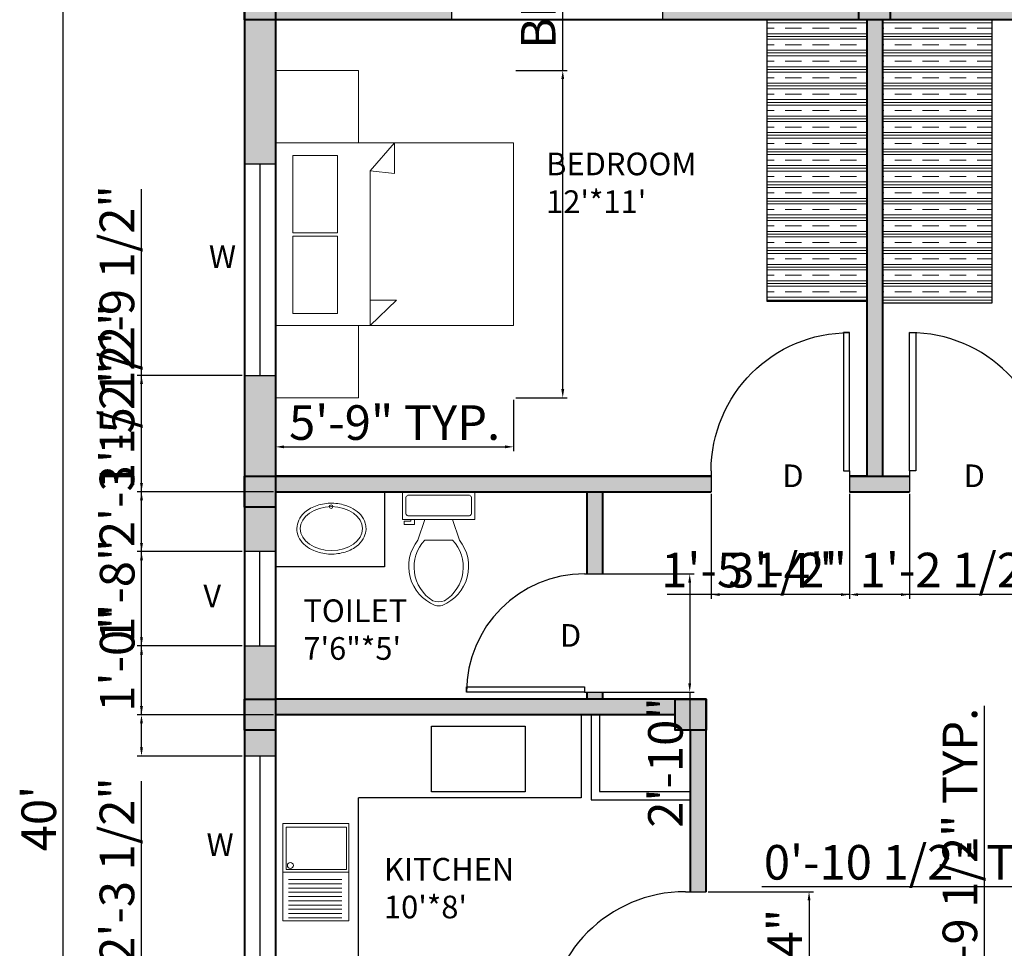
# Model space of a CAD drawing. Units: inches. Extents: x 1628 to 2197, y 2073 to 2736.
# Tile 2 of 3: x 1628 to 1913, y 2323 to 2592. Entities that reach past the tile are written whole.
import ezdxf

# ---------------------------------------------------------------- set-up
doc = ezdxf.new("R2010")
doc.units = ezdxf.units.IN
for name, color, linetype, lineweight in [('A-ANNO-DIMS', 2, 'Continuous', 18), ('A-ANNO-IDEN', 7, 'Continuous', 18), ('A-AREA-IDEN', 7, 'Continuous', 18), ('A-COLS', 7, 'Continuous', 40), ('A-COLS-PATT', 8, 'Continuous', 13), ('A-FLOR-CASE', 8, 'Continuous', 25), ('A-FLOR-CASE-PATT', 9, 'Continuous', 13), ('A-FLOR-FIXT', 8, 'Continuous', 18), ('A-FLOR-FIXT-PATT', 8, 'Continuous', 13), ('A-WALL-PATT', 152, 'Continuous', 13), ('bed', 210, 'Continuous', 18), ('door', 52, 'Continuous', 25), ('wall', 151, 'Continuous', 40), ('window', 20, 'Continuous', 25)]:
    doc.layers.add(name, color=color, linetype=linetype, lineweight=lineweight)
doc.styles.get("Standard").update_dxf_attribs({"font": 'arial.ttf'})
doc.dimstyles.new('ISO-25', dxfattribs={"dimtxt": 10, "dimasz": 2.5, "dimexe": 1.25, "dimexo": 0.625, "dimtad": 1, "dimdec": 0, "dimlunit": 4, "dimtxsty": 'Standard', "dimcen": 2.5, "dimadec": 0, "dimazin": 0, "dimtfac": 1, "dimtdec": 0, "dimtmove": 0, "dimatfit": 3, "dimfxl": 1, "dimarcsym": 0})

# ---------------------------------------------------------------- blocks, each defined once
blk = doc.blocks.new('*U2')
for p, q in [((0, 0), (-1e-16, -5.999999999999999)), ((40, -6e-16), (40, -6))]:
    blk.add_line(p, q)
blk.add_lwpolyline([(0, 0), (5.6e-15, 40), (1.750000000000007, 40), (1.749999999999998, -7e-16)], close=True)
blk.add_arc((0, 0), 40, 0, 90)
blk = doc.blocks.new('*U4')
for p, q in [((9.5, -6), (9.5, -2)), ((-10, -8.5), (-8, -8.5)), ((-10, -9.5), (-10, -8.5)), ((-8, -8.5), (-8, -8)), ((-7, -8), (-7, -9.5)), ((-4, -8), (-6, -14)), ((4, -8), (6, -14)), ((-7, -9.5), (-10, -9.5)), ((4, -14), (-4, -14))]:
    blk.add_line(p, q)
blk.add_lwpolyline([(10.5, -8), (10.5, 0), (-10.5, 0), (-10.5, -8)], close=True)
for points in [[(-9.5, -2), (-9.5, -6)], [(8.5, -1), (-8.5, -1)], [(-8.5, -7), (8.5, -7)]]:
    blk.add_lwpolyline(points)
for centre, radius, start, end in [((-8.625, -1.875), 0.8838834999999999, 81.86989999999999, 188.1300999999999), ((8.625, -1.875), 0.8838834999999999, 351.8699, 98.13009999999993), ((-8.625, -6.125), 0.8838834999999999, 171.869898, 278.1301), ((8.625, -6.125), 0.8838834999999999, 261.8699, 8.130099999999993), ((3.519562435188956, -21.58049502388982), 12.16902005083646, 141.4691096810948, 247.9714346835576), ((4.199957580658807, -21.81740929088453), 11.3291791325804, 136.3677254423718, 238.946823937405), ((-3.519499936778316, -21.58047137067522), 12.16903423757823, 292.0284332733152, 38.53070636800453), ((-4.199890672038477, -21.81738596564128), 11.32918622148567, 301.0530065773863, 43.63209216694732), ((2.09660981727e-05, -27.87646475467881), 4, 245.7318247449371, 294.2681740488959), ((2.09415214183e-05, -28.99996806116075), 4, 254.8605283244437, 285.1394707718433)]:
    blk.add_arc(centre, radius, start, end)
blk = doc.blocks.new('*D6')
at = {"layer": 'A-ANNO-DIMS', "color": 0, "lineweight": -2, "transparency": 16777216}
for p, q in [((1692.485896843686, 2600.702398616904), (1639.445355811252, 2600.702398616904)), ((1640.695355811253, 2123.202398616904), (1640.695355811252, 2598.202398616904)), ((1692.485896843686, 2120.702398616904), (1639.445355811253, 2120.702398616904))]:
    blk.add_line(p, q, dxfattribs=at)
at = {"layer": 'A-ANNO-DIMS', "color": 0, "transparency": 16777216}
for points in [[(1640.278689144586, 2598.202398616904), (1641.112022477919, 2598.202398616904), (1640.695355811252, 2600.702398616904)], [(1640.278689144586, 2123.202398616904), (1641.112022477919, 2123.202398616904), (1640.695355811253, 2120.702398616904)]]:
    blk.add_solid(points, dxfattribs=at)
at = {"layer": 'Defpoints', "color": 0, "transparency": 16777216}
for p in [(1640.695355811252, 2600.702398616904), (1693.110896843687, 2600.702398616904), (1693.110896843687, 2120.702398616904)]:
    blk.add_point(p, dxfattribs=at)
at = {"layer": 'A-ANNO-DIMS', "color": 0, "transparency": 16777216, "insert": (1634.964625934036, 2360.702398616903), "char_height": 10, "attachment_point": 5, "rotation": 90}
blk.add_mtext("40'", dxfattribs=at)
blk = doc.blocks.new('BED-DOUBLE-WITH-NIGHTSTANDS')
for p, q in [((27.36977918091793, 65.5958310632277), (34.42114521002327, 73.72468310128534)), ((34.42114521002327, 73.72468310128534), (34.42114521002327, 64.85614303712828)), ((27.36977918091793, 28.24148243144555), (27.36977918091793, 65.5958310632277)), ((34.42114521002327, 64.85614303712828), (27.36977918091793, 65.5958310632277)), ((27.36977918091793, 28.24148243144555), (27.36977918091793, 20.93786224134965)), ((27.36977918091793, 20.93786224134965), (34.95813081485972, 28.24148243144555)), ((34.95813081485972, 28.24148243144555), (27.36977918091793, 28.24148243144555))]:
    blk.add_line(p, q)
for points in [[(-0.0001031563144807, 73.72468310128534), (23.97928037784254, 73.72468310128534), (23.97928037784254, 94.66247624076277), (-0.0001031563144807, 94.66247624076277)], [(-0.0001031563144807, 20.93786224134965), (68.84239357636102, 20.93786224134965), (68.84239357636102, 73.72468310128534), (-0.0001031563144807, 73.72468310128534)], [(4.974907084450705, 47.65834800199082), (17.93062219200033, 47.65834800199082), (17.93062219200033, 70.03397213404423), (4.974907084450705, 70.03397213404423)], [(4.974907084450705, 24.35811060875858), (17.93062219200033, 24.35811060875858), (17.93062219200033, 46.73373474081199), (4.974907084450705, 46.73373474081199)], [(-0.0001031563144807, 6.91018722137e-05), (23.97928037784254, 6.91018722137e-05), (23.97928037784254, 20.93786224134965), (-0.0001031563144807, 20.93786224134965)]]:
    blk.add_lwpolyline(points, close=True)
blk = doc.blocks.new('WINDOW-61IN')
blk.add_line((-0.0003684333103138, 4.500398616903112), (61.10273973038352, 4.500398616903112))
blk.add_lwpolyline([(-0.0003684333103138, 0.0003986169031123), (61.10273973038352, 0.0003986169031123), (61.10273973038352, 9.000398616903112), (-0.0003684333103138, 9.000398616903112)], close=True)
blk = doc.blocks.new('COLUMN-9X9')
blk.add_lwpolyline([(-0.0001031563144807, 9.000398616903112), (8.99989684368552, 9.000398616903112), (8.99989684368552, 0.0003986169031123), (-0.0001031563144807, 0.0003986169031123)], close=True)
blk = doc.blocks.new('*D18')
at = {"layer": 'A-ANNO-DIMS', "color": 0, "lineweight": -2, "transparency": 16777216}
for p, q in [((1938.501053468832, 2340.938171535931), (1842.725132595708, 2340.938171535927)), ((1938.501053468832, 2342.288259422146), (1938.501053468832, 2339.688171535931)), ((1946.605665621899, 2340.938171535931), (1941.001053468832, 2340.938171535931)), ((1949.1056656219, 2342.288259422147), (1949.1056656219, 2339.688171535931))]:
    blk.add_line(p, q, dxfattribs=at)
at = {"layer": 'A-ANNO-DIMS', "color": 0, "transparency": 16777216}
for points in [[(1941.001053468832, 2341.354838202597), (1941.001053468832, 2340.521504869264), (1938.501053468832, 2340.938171535931)], [(1946.605665621899, 2341.354838202597), (1946.605665621899, 2340.521504869264), (1949.1056656219, 2340.938171535931)]]:
    blk.add_solid(points, dxfattribs=at)
at = {"layer": 'Defpoints', "color": 0, "transparency": 16777216}
for p in [(1938.501053468832, 2342.913259422146), (1949.1056656219, 2342.913259422147), (1938.501053468832, 2340.938171535931)]:
    blk.add_point(p, dxfattribs=at)
at = {"layer": 'A-ANNO-DIMS', "color": 0, "transparency": 16777216, "insert": (1889.36309303227, 2346.733703595956), "char_height": 10, "attachment_point": 5}
blk.add_mtext('0\'-10 1/2" TYP.', dxfattribs=at)
blk = doc.blocks.new('*D19')
at = {"layer": 'A-ANNO-DIMS', "color": 0, "lineweight": -2, "transparency": 16777216}
for p, q in [((1785.152754647198, 2577.035625777927), (1785.152754647198, 2736.024370661965)), ((1771.578393576364, 2577.035625777927), (1786.402754647198, 2577.035625777927)), ((1785.152754647198, 2484.873218639036), (1785.152754647198, 2574.535625777927)), ((1771.578393576364, 2482.373218639037), (1786.402754647198, 2482.373218639037))]:
    blk.add_line(p, q, dxfattribs=at)
at = {"layer": 'A-ANNO-DIMS', "color": 0, "transparency": 16777216}
for points in [[(1784.736087980531, 2574.535625777927), (1785.569421313865, 2574.535625777927), (1785.152754647198, 2577.035625777927)], [(1784.736087980532, 2484.873218639036), (1785.569421313865, 2484.873218639036), (1785.152754647198, 2482.373218639037)]]:
    blk.add_solid(points, dxfattribs=at)
at = {"layer": 'Defpoints', "color": 0, "transparency": 16777216}
for p in [(1770.953393576364, 2577.035625777927), (1785.152754647198, 2577.035625777927), (1770.953393576364, 2482.373218639037)]:
    blk.add_point(p, dxfattribs=at)
at = {"layer": 'A-ANNO-DIMS', "color": 0, "transparency": 16777216, "insert": (1779.357222587171, 2657.779998219945), "char_height": 10, "attachment_point": 5, "rotation": 90}
blk.add_mtext('BED SET 7\'-10 1/2" TYP.', dxfattribs=at)
blk = doc.blocks.new('*D20')
at = {"layer": 'A-ANNO-DIMS', "color": 0, "lineweight": -2, "transparency": 16777216}
for p, q in [((1702.110896843687, 2481.748218639035), (1702.110896843687, 2466.923857568202)), ((1770.953393576363, 2481.748218639035), (1770.953393576363, 2466.923857568202)), ((1704.610896843687, 2468.173857568201), (1768.453393576363, 2468.173857568201))]:
    blk.add_line(p, q, dxfattribs=at)
at = {"layer": 'A-ANNO-DIMS', "color": 0, "transparency": 16777216}
for points in [[(1704.610896843687, 2468.590524234868), (1704.610896843687, 2467.757190901535), (1702.110896843687, 2468.173857568201)], [(1768.453393576363, 2468.590524234868), (1768.453393576363, 2467.757190901535), (1770.953393576363, 2468.173857568201)]]:
    blk.add_solid(points, dxfattribs=at)
at = {"layer": 'Defpoints', "color": 0, "transparency": 16777216}
for p in [(1702.110896843687, 2482.373218639035), (1770.953393576363, 2482.373218639035), (1770.953393576363, 2468.173857568201)]:
    blk.add_point(p, dxfattribs=at)
at = {"layer": 'A-ANNO-DIMS', "color": 0, "transparency": 16777216, "insert": (1736.532145210025, 2473.904587445419), "char_height": 10, "attachment_point": 5}
blk.add_mtext('5\'-9" TYP.', dxfattribs=at)
blk = doc.blocks.new('*D24')
at = {"layer": 'A-ANNO-DIMS', "color": 0, "lineweight": -2, "transparency": 16777216}
for p, q in [((1907.071103678795, 2305.097810115476), (1907.071103678795, 2393.274822393784)), ((1916.945934926503, 2305.097810115476), (1905.821103678795, 2305.097810115476)), ((1907.071103678795, 2274.241064235891), (1907.071103678795, 2302.597810115477)), ((1916.945934926503, 2271.741064235891), (1905.821103678795, 2271.741064235891))]:
    blk.add_line(p, q, dxfattribs=at)
at = {"layer": 'A-ANNO-DIMS', "color": 0, "transparency": 16777216}
for points in [[(1906.654437012129, 2302.597810115477), (1907.487770345462, 2302.597810115477), (1907.071103678795, 2305.097810115476)], [(1906.654437012129, 2274.241064235891), (1907.487770345462, 2274.241064235891), (1907.071103678795, 2271.741064235891)]]:
    blk.add_solid(points, dxfattribs=at)
at = {"layer": 'Defpoints', "color": 0, "transparency": 16777216}
for p in [(1907.071103678795, 2305.097810115476), (1917.570934926503, 2305.097810115476), (1917.570934926503, 2271.741064235891)]:
    blk.add_point(p, dxfattribs=at)
at = {"layer": 'A-ANNO-DIMS', "color": 0, "transparency": 16777216, "insert": (1901.275571618768, 2350.43631625463), "char_height": 10, "attachment_point": 5, "rotation": 90}
blk.add_mtext('2\'-9 1/2" TYP.', dxfattribs=at)
blk = doc.blocks.new('*D35')
at = {"layer": 'A-ANNO-DIMS', "color": 0, "lineweight": -2, "transparency": 16777216}
for p, q in [((1663.360897000002, 2317.649085000001), (1663.360897000002, 2371.45365525921)), ((1692.485897000001, 2317.649085000001), (1662.110897000002, 2317.649085000001)), ((1663.360897000002, 2292.702399000001), (1663.360897000002, 2315.149085000001)), ((1701.485897000001, 2290.202399000001), (1662.110897000002, 2290.202399000001))]:
    blk.add_line(p, q, dxfattribs=at)
at = {"layer": 'A-ANNO-DIMS', "color": 0, "transparency": 16777216}
for points in [[(1662.944230333335, 2315.149085000001), (1663.777563666668, 2315.149085000001), (1663.360897000002, 2317.649085000001)], [(1662.944230333335, 2292.702399000001), (1663.777563666668, 2292.702399000001), (1663.360897000002, 2290.202399000001)]]:
    blk.add_solid(points, dxfattribs=at)
at = {"layer": 'Defpoints', "color": 0, "transparency": 16777216}
for p in [(1663.360897000002, 2317.649085000001), (1693.110897000001, 2317.649085000001), (1702.110897000001, 2290.202399000001)]:
    blk.add_point(p, dxfattribs=at)
at = {"layer": 'A-ANNO-DIMS', "color": 0, "transparency": 16777216, "insert": (1657.561954298774, 2345.801370129604), "char_height": 10, "attachment_point": 5, "rotation": 90}
blk.add_mtext('2\'-3 1/2"', dxfattribs=at)
blk = doc.blocks.new('*D36')
at = {"layer": 'A-ANNO-DIMS', "color": 0, "lineweight": -2, "transparency": 16777216}
for p, q in [((1663.360897000002, 2390.702399000001), (1663.360897000002, 2420.093599545703)), ((1701.485897000001, 2390.702399000001), (1662.110897000002, 2390.702399000001)), ((1663.360897000002, 2381.252193000001), (1663.360897000002, 2388.202399000001)), ((1692.485897000001, 2378.752193000001), (1662.110897000002, 2378.752193000001))]:
    blk.add_line(p, q, dxfattribs=at)
at = {"layer": 'A-ANNO-DIMS', "color": 0, "transparency": 16777216}
for points in [[(1662.944230333335, 2388.202399000001), (1663.777563666668, 2388.202399000001), (1663.360897000002, 2390.702399000001)], [(1662.944230333335, 2381.252193000001), (1663.777563666668, 2381.252193000001), (1663.360897000002, 2378.752193000001)]]:
    blk.add_solid(points, dxfattribs=at)
at = {"layer": 'Defpoints', "color": 0, "transparency": 16777216}
for p in [(1663.360897000002, 2390.702399000001), (1702.110897000001, 2390.702399000001), (1693.110897000001, 2378.752193000001)]:
    blk.add_point(p, dxfattribs=at)
at = {"layer": 'A-ANNO-DIMS', "color": 0, "transparency": 16777216, "insert": (1657.630167122785, 2406.647999272851), "char_height": 10, "attachment_point": 5, "rotation": 90}
blk.add_mtext('1\'-0"', dxfattribs=at)
blk = doc.blocks.new('*D37')
at = {"layer": 'A-ANNO-DIMS', "color": 0, "lineweight": -2, "transparency": 16777216}
for p, q in [((1663.360897000002, 2410.599066000001), (1663.360897000002, 2439.990266545704)), ((1692.485897000001, 2410.599066000001), (1662.110897000002, 2410.599066000001)), ((1663.360897000002, 2393.202399000001), (1663.360897000002, 2408.099066000001)), ((1701.485897000001, 2390.702399000001), (1662.110897000002, 2390.702399000001))]:
    blk.add_line(p, q, dxfattribs=at)
at = {"layer": 'A-ANNO-DIMS', "color": 0, "transparency": 16777216}
for points in [[(1662.944230333335, 2408.099066000001), (1663.777563666668, 2408.099066000001), (1663.360897000002, 2410.599066000001)], [(1662.944230333335, 2393.202399000001), (1663.777563666668, 2393.202399000001), (1663.360897000002, 2390.702399000001)]]:
    blk.add_solid(points, dxfattribs=at)
at = {"layer": 'Defpoints', "color": 0, "transparency": 16777216}
for p in [(1663.360897000002, 2410.599066000001), (1693.110897000001, 2410.599066000001), (1702.110897000001, 2390.702399000001)]:
    blk.add_point(p, dxfattribs=at)
at = {"layer": 'A-ANNO-DIMS', "color": 0, "transparency": 16777216, "insert": (1657.630167122785, 2426.544666272852), "char_height": 10, "attachment_point": 5, "rotation": 90}
blk.add_mtext('1\'-8"', dxfattribs=at)
blk = doc.blocks.new('*D38')
at = {"layer": 'A-ANNO-DIMS', "color": 0, "lineweight": -2, "transparency": 16777216}
for p, q in [((1663.360897000002, 2437.863608000001), (1663.360897000002, 2491.66817825921)), ((1692.485897000001, 2437.863608000001), (1662.110897000002, 2437.863608000001)), ((1663.360897000002, 2413.099066000001), (1663.360897000002, 2435.363608000001)), ((1692.485897000001, 2410.599066000001), (1662.110897000002, 2410.599066000001))]:
    blk.add_line(p, q, dxfattribs=at)
at = {"layer": 'A-ANNO-DIMS', "color": 0, "transparency": 16777216}
for points in [[(1662.944230333335, 2435.363608000001), (1663.777563666668, 2435.363608000001), (1663.360897000002, 2437.863608000001)], [(1662.944230333335, 2413.099066000001), (1663.777563666668, 2413.099066000001), (1663.360897000002, 2410.599066000001)]]:
    blk.add_solid(points, dxfattribs=at)
at = {"layer": 'Defpoints', "color": 0, "transparency": 16777216}
for p in [(1663.360897000002, 2437.863608000001), (1693.110897000001, 2437.863608000001), (1693.110897000001, 2410.599066000001)]:
    blk.add_point(p, dxfattribs=at)
at = {"layer": 'A-ANNO-DIMS', "color": 0, "transparency": 16777216, "insert": (1657.561954298774, 2466.015893129605), "char_height": 10, "attachment_point": 5, "rotation": 90}
blk.add_mtext('2\'-3 1/2"', dxfattribs=at)
blk = doc.blocks.new('*D39')
at = {"layer": 'A-ANNO-DIMS', "color": 0, "lineweight": -2, "transparency": 16777216}
for p, q in [((1663.360897000002, 2455.202399000001), (1663.360897000002, 2507.895100227831)), ((1701.485897000001, 2455.202399000001), (1662.110897000002, 2455.202399000001)), ((1663.360897000002, 2440.363608000001), (1663.360897000002, 2452.702399000001)), ((1692.485897000001, 2437.863608000001), (1662.110897000002, 2437.863608000001))]:
    blk.add_line(p, q, dxfattribs=at)
at = {"layer": 'A-ANNO-DIMS', "color": 0, "transparency": 16777216}
for points in [[(1662.944230333335, 2452.702399000001), (1663.777563666668, 2452.702399000001), (1663.360897000002, 2455.202399000001)], [(1662.944230333335, 2440.363608000001), (1663.777563666668, 2440.363608000001), (1663.360897000002, 2437.863608000001)]]:
    blk.add_solid(points, dxfattribs=at)
at = {"layer": 'Defpoints', "color": 0, "transparency": 16777216}
for p in [(1663.360897000002, 2455.202399000001), (1702.110897000001, 2455.202399000001), (1693.110897000001, 2437.863608000001)]:
    blk.add_point(p, dxfattribs=at)
at = {"layer": 'A-ANNO-DIMS', "color": 0, "transparency": 16777216, "insert": (1657.565364939975, 2482.798749613916), "char_height": 10, "attachment_point": 5, "rotation": 90}
blk.add_mtext('1\'-5 1/2"', dxfattribs=at)
blk = doc.blocks.new('*D40')
at = {"layer": 'A-ANNO-DIMS', "color": 0, "lineweight": -2, "transparency": 16777216}
for p, q in [((1663.360897000002, 2488.850109000001), (1663.360897000002, 2542.65467925921)), ((1692.485897000001, 2488.850109000001), (1662.110897000002, 2488.850109000001)), ((1663.360897000002, 2457.702399000001), (1663.360897000002, 2486.350109000001)), ((1701.485897000001, 2455.202399000001), (1662.110897000002, 2455.202399000001))]:
    blk.add_line(p, q, dxfattribs=at)
at = {"layer": 'A-ANNO-DIMS', "color": 0, "transparency": 16777216}
for points in [[(1662.944230333335, 2486.350109000001), (1663.777563666668, 2486.350109000001), (1663.360897000002, 2488.850109000001)], [(1662.944230333335, 2457.702399000001), (1663.777563666668, 2457.702399000001), (1663.360897000002, 2455.202399000001)]]:
    blk.add_solid(points, dxfattribs=at)
at = {"layer": 'Defpoints', "color": 0, "transparency": 16777216}
for p in [(1663.360897000002, 2488.850109000001), (1693.110897000001, 2488.850109000001), (1702.110897000001, 2455.202399000001)]:
    blk.add_point(p, dxfattribs=at)
at = {"layer": 'A-ANNO-DIMS', "color": 0, "transparency": 16777216, "insert": (1657.565364939975, 2517.002394129605), "char_height": 10, "attachment_point": 5, "rotation": 90}
blk.add_mtext('2\'-9 1/2"', dxfattribs=at)
blk = doc.blocks.new('*D48')
at = {"layer": 'A-ANNO-DIMS', "color": 0, "lineweight": -2, "transparency": 16777216}
for p, q in [((1792.735897000001, 2431.437917000002), (1823.110897000002, 2431.437917000002)), ((1821.860897000002, 2428.937917000001), (1821.860897000002, 2399.766059000001)), ((1792.735897000001, 2397.266059000001), (1823.110897000002, 2397.266059000001)), ((1821.860897000002, 2397.266059000001), (1821.860897000002, 2358.993548768077))]:
    blk.add_line(p, q, dxfattribs=at)
at = {"layer": 'A-ANNO-DIMS', "color": 0, "transparency": 16777216}
for points in [[(1821.444230333335, 2428.937917000001), (1822.277563666668, 2428.937917000001), (1821.860897000002, 2431.437917000002)], [(1821.444230333335, 2399.766059000001), (1822.277563666668, 2399.766059000001), (1821.860897000002, 2397.266059000001)]]:
    blk.add_solid(points, dxfattribs=at)
at = {"layer": 'Defpoints', "color": 0, "transparency": 16777216}
for p in [(1792.110897000001, 2431.437917000002), (1792.110897000001, 2397.266059000001), (1821.860897000002, 2397.266059000001)]:
    blk.add_point(p, dxfattribs=at)
at = {"layer": 'A-ANNO-DIMS', "color": 0, "transparency": 16777216, "insert": (1816.130167122785, 2376.879803884039), "char_height": 10, "attachment_point": 5, "rotation": 90}
blk.add_mtext('2\'-10"', dxfattribs=at)
blk = doc.blocks.new('*D49')
at = {"layer": 'A-ANNO-DIMS', "color": 0, "lineweight": -2, "transparency": 16777216}
for p, q in [((1828.052739, 2454.577399), (1828.052739, 2424.202399)), ((1868.052739, 2454.577399), (1868.052739, 2424.202399)), ((1865.552739, 2425.452399), (1830.552739, 2425.452399))]:
    blk.add_line(p, q, dxfattribs=at)
at = {"layer": 'A-ANNO-DIMS', "color": 0, "transparency": 16777216}
for points in [[(1830.552739, 2425.869065666666), (1830.552739, 2425.035732333333), (1828.052739, 2425.452399)], [(1865.552739, 2425.869065666666), (1865.552739, 2425.035732333333), (1868.052739, 2425.452399)]]:
    blk.add_solid(points, dxfattribs=at)
at = {"layer": 'Defpoints', "color": 0, "transparency": 16777216}
for p in [(1828.052739, 2455.202399), (1868.052739, 2455.202399), (1828.052739, 2425.452399)]:
    blk.add_point(p, dxfattribs=at)
at = {"layer": 'A-ANNO-DIMS', "color": 0, "transparency": 16777216, "insert": (1848.052739, 2431.186539518418), "char_height": 10, "attachment_point": 5}
blk.add_mtext('3\'-4"', dxfattribs=at)
blk = doc.blocks.new('*D50')
at = {"layer": 'A-ANNO-DIMS', "color": 0, "lineweight": -2, "transparency": 16777216}
for p, q in [((1868.052739, 2454.577399), (1868.052739, 2424.202399)), ((1885.432438, 2454.577399), (1885.432438, 2424.202399)), ((1868.052739, 2425.452399), (1815.360037772169, 2425.452399)), ((1882.932438, 2425.452399), (1870.552739, 2425.452399))]:
    blk.add_line(p, q, dxfattribs=at)
at = {"layer": 'A-ANNO-DIMS', "color": 0, "transparency": 16777216}
for points in [[(1870.552739, 2425.869065666666), (1870.552739, 2425.035732333333), (1868.052739, 2425.452399)], [(1882.932438, 2425.869065666666), (1882.932438, 2425.035732333333), (1885.432438, 2425.452399)]]:
    blk.add_solid(points, dxfattribs=at)
at = {"layer": 'Defpoints', "color": 0, "transparency": 16777216}
for p in [(1868.052739, 2455.202399), (1885.432438, 2455.202399), (1868.052739, 2425.452399)]:
    blk.add_point(p, dxfattribs=at)
at = {"layer": 'A-ANNO-DIMS', "color": 0, "transparency": 16777216, "insert": (1840.456388386084, 2431.247931060027), "char_height": 10, "attachment_point": 5}
blk.add_mtext('1\'-5 1/2"', dxfattribs=at)
blk = doc.blocks.new('*D51')
at = {"layer": 'A-ANNO-DIMS', "color": 0, "lineweight": -2, "transparency": 16777216}
for p, q in [((1925.432438, 2454.577399), (1925.432437999998, 2424.202399)), ((1940.110897, 2454.577399), (1940.110896999998, 2424.202398999999)), ((1925.432437999998, 2425.452399), (1872.739736772167, 2425.452399000004)), ((1937.610896999998, 2425.452399), (1927.932437999998, 2425.452399))]:
    blk.add_line(p, q, dxfattribs=at)
at = {"layer": 'A-ANNO-DIMS', "color": 0, "transparency": 16777216}
for points in [[(1927.932437999998, 2425.869065666666), (1927.932437999998, 2425.035732333333), (1925.432437999998, 2425.452399)], [(1937.610896999998, 2425.869065666666), (1937.610896999998, 2425.035732333333), (1940.110896999998, 2425.452399)]]:
    blk.add_solid(points, dxfattribs=at)
at = {"layer": 'Defpoints', "color": 0, "transparency": 16777216}
for p in [(1925.432438, 2455.202399), (1940.110897, 2455.202399), (1925.432437999998, 2425.452399)]:
    blk.add_point(p, dxfattribs=at)
at = {"layer": 'A-ANNO-DIMS', "color": 0, "transparency": 16777216, "insert": (1897.836087386083, 2431.247931060029), "char_height": 10, "attachment_point": 5}
blk.add_mtext('1\'-2 1/2"', dxfattribs=at)
blk = doc.blocks.new('*D53')
at = {"layer": 'A-ANNO-DIMS', "color": 0, "lineweight": -2, "transparency": 16777216}
for p, q in [((1827.235897000001, 2339.518037000001), (1857.610897000002, 2339.518037000001)), ((1856.360897000002, 2337.018037000001), (1856.360897000002, 2302.018037000001)), ((1827.235897000001, 2299.518037000001), (1857.610897000002, 2299.518037000001))]:
    blk.add_line(p, q, dxfattribs=at)
at = {"layer": 'A-ANNO-DIMS', "color": 0, "transparency": 16777216}
for points in [[(1855.944230333335, 2337.018037000001), (1856.777563666668, 2337.018037000001), (1856.360897000002, 2339.518037000001)], [(1855.944230333335, 2302.018037000001), (1856.777563666668, 2302.018037000001), (1856.360897000002, 2299.518037000001)]]:
    blk.add_solid(points, dxfattribs=at)
at = {"layer": 'Defpoints', "color": 0, "transparency": 16777216}
for p in [(1826.610897000001, 2339.518037000001), (1826.610897000001, 2299.518037000001), (1856.360897000002, 2299.518037000001)]:
    blk.add_point(p, dxfattribs=at)
at = {"layer": 'A-ANNO-DIMS', "color": 0, "transparency": 16777216, "insert": (1850.626756481585, 2319.518037), "char_height": 10, "attachment_point": 5, "rotation": 90}
blk.add_mtext('3\'-4"', dxfattribs=at)

msp = doc.modelspace()

# ---------------------------------------------------------------- hatches: boundary and pattern name
at = {"layer": 'A-COLS-PATT'}
h = msp.add_hatch(color=256, dxfattribs=at)
h.dxf.hatch_style = 1
h.paths.add_polyline_path([(1702.110896843685, 2600.702398616903), (1693.110896843685, 2600.702398616903), (1693.110896843685, 2591.702398616904), (1702.110896843685, 2591.702398616904)])
h.paths.add_polyline_path([(1879.789544656754, 2600.702398616903), (1870.789544656754, 2600.702398616903), (1870.789544656754, 2591.702398616904), (1879.789544656754, 2591.702398616904)])
h.paths.add_polyline_path([(2053.110896843686, 2600.702398616903), (2044.110896843686, 2600.702398616903), (2044.110896843686, 2591.702398616904), (2053.110896843686, 2591.702398616904)])
h.paths.add_polyline_path([(1702.110896843685, 2395.202398616904), (1693.110896843685, 2395.202398616904), (1693.110896843685, 2386.202398616903), (1702.110896843685, 2386.202398616903)])
h.paths.add_polyline_path([(1826.610896843686, 2395.202398616904), (1817.610896843685, 2395.202398616904), (1817.610896843685, 2386.202398616903), (1826.610896843686, 2386.202398616903)])
h.paths.add_polyline_path([(1702.110896843685, 2459.702398616903), (1693.110896843685, 2459.702398616903), (1693.110896843685, 2450.702398616904), (1702.110896843685, 2450.702398616904)])
h.paths.add_polyline_path([(2053.110896843686, 2459.702398616903), (2044.110896843686, 2459.702398616903), (2044.110896843686, 2455.202398616903), (2053.110896843686, 2455.202398616903)])
h.paths.add_polyline_path([(2053.110896843686, 2455.202398616903), (2044.110896843686, 2455.202398616903), (2044.110896843686, 2451.940390996), (2053.110896843686, 2451.940390996)])
h.paths.add_polyline_path([(2053.110896843686, 2460.940390996), (2044.110896843686, 2460.940390996), (2044.110896843686, 2459.702398616903), (2053.110896843686, 2459.702398616903)])
h.paths.add_polyline_path([(2053.110896843686, 2390.990533735672), (2044.110896843686, 2390.990533735672), (2044.110896843686, 2381.990533735671), (2053.110896843686, 2381.990533735671)])
h.paths.add_polyline_path([(2053.110896843686, 2322.517334083322), (2044.110896843686, 2322.517334083322), (2044.110896843686, 2313.517334083321), (2053.110896843686, 2313.517334083321)])
h.paths.add_polyline_path([(1702.110896843685, 2294.702398616903), (1693.110896843685, 2294.702398616903), (1693.110896843685, 2285.702398616903), (1702.110896843685, 2285.702398616903)])
h.paths.add_polyline_path([(1702.110896843685, 2129.702398616903), (1693.110896843685, 2129.702398616903), (1693.110896843685, 2120.702398616904), (1702.110896843685, 2120.702398616904)])
h.paths.add_polyline_path([(1831.350600622014, 2129.702398616903), (1822.350600622014, 2129.702398616903), (1822.350600622014, 2120.702398616904), (1831.350600622014, 2120.702398616904)])
h.paths.add_polyline_path([(1883.720266620277, 2129.702398616903), (1874.720266620277, 2129.702398616903), (1874.720266620277, 2120.702398616904), (1883.720266620277, 2120.702398616904)])
h.paths.add_polyline_path([(2053.110896843686, 2129.702398616903), (2044.110896843686, 2129.702398616903), (2044.110896843686, 2120.702398616904), (2053.110896843686, 2120.702398616904)])
at = {"layer": 'A-FLOR-CASE-PATT'}
h = msp.add_hatch(dxfattribs=at)
h.set_pattern_fill('CLAY', color=256)
h.set_pattern_definition([(0, (0, 0), (0, 4.7625), []), (0, (0, 0.79375), (0, 4.7625), []), (0, (0, 1.587499999999999), (0, 4.7625), []), (0, (0, 3.174999999999999), (0, 4.7625), [4.7625, -3.174999999999999])])
h.paths.add_polyline_path([(1873.110896843686, 2591.702398616904), (1844.252398980434, 2591.702398616904), (1844.252398980434, 2510.242728136783), (1873.110896843686, 2510.242728136783)])
h.paths.add_polyline_path([(1909.320134716665, 2591.702398616904), (1877.610896843685, 2591.702398616904), (1877.610896843685, 2509.82863999123), (1909.320134716665, 2509.82863999123)])
at = {"layer": 'A-FLOR-FIXT-PATT'}
h = msp.add_hatch(dxfattribs=at)
h.set_pattern_fill('ANSI31', color=256, scale=0.386166, angle=-45, style=0)
h.set_pattern_definition([(0, (0, 0), (0, 1.22607705), [])])
h.paths.add_polyline_path([(1705.896944, 2331.99642), (1721.236081, 2331.99642), (1721.236081, 2344.176245), (1705.896944, 2344.176245)])
at = {"layer": 'A-WALL-PATT'}
h = msp.add_hatch(color=256, dxfattribs=at)
h.dxf.hatch_style = 1
h.paths.add_polyline_path([(1753.013631566689, 2600.702398616903), (1702.110896843685, 2600.702398616903), (1702.110896843685, 2591.702398616904), (1753.013631566689, 2591.702398616904)])
h.paths.add_polyline_path([(1870.789544656754, 2600.702398616903), (1814.116739730383, 2600.702398616903), (1814.116739730383, 2591.702398616904), (1870.789544656754, 2591.702398616904)])
h.paths.add_polyline_path([(1948.368746460448, 2600.702398616903), (1879.789544656754, 2600.702398616903), (1879.789544656754, 2591.702398616904), (1909.320134716665, 2591.702398616904), (1948.368746460448, 2591.702398616904)])
h.paths.add_polyline_path([(2044.110896843686, 2600.702398616903), (2009.471854624142, 2600.702398616903), (2009.471854624142, 2591.702398616904), (2044.110896843686, 2591.702398616904)])
h.paths.add_polyline_path([(2053.110896843686, 2591.702398616904), (2044.110896843686, 2591.702398616904), (2044.110896843686, 2550.072421842385), (2053.110896843686, 2550.072421842385)])
h.paths.add_polyline_path([(1702.110896843685, 2591.702398616904), (1693.110896843685, 2591.702398616904), (1693.110896843685, 2549.953217094844), (1702.110896843685, 2549.953217094844)])
h.paths.add_polyline_path([(1702.110896843685, 2488.85010893115), (1693.110896843685, 2488.85010893115), (1693.110896843685, 2459.702398616903), (1702.110896843685, 2459.702398616903)])
h.paths.add_polyline_path([(1828.052739298115, 2459.702398616904), (1702.110896843685, 2459.702398616903), (1702.110896843685, 2455.202398616903), (1733.607219099031, 2455.202398616903), (1792.110896843686, 2455.202398616903), (1828.052739298115, 2455.202398616904)])
h.paths.add_polyline_path([(1885.432437777228, 2459.702398616904), (1868.052739298114, 2459.702398616904), (1868.052739298114, 2455.202398616904), (1885.432437777228, 2455.202398616904)])
h.paths.add_polyline_path([(2053.110896843686, 2488.969313678691), (2044.110896843686, 2488.969313678691), (2044.110896843686, 2474.676024548712), (2044.110896843686, 2460.940390996), (2053.110896843686, 2460.940390996)])
h.paths.add_polyline_path([(2053.110896843686, 2451.940390996), (2044.110896843686, 2451.940390996), (2044.110896843686, 2437.286361970541), (2053.110896843686, 2437.286361970541)])
h.paths.add_polyline_path([(2053.110896843686, 2414.882591286594), (2044.110896843686, 2414.882591286594), (2044.110896843686, 2390.990533735672), (2053.110896843686, 2390.990533735672)])
h.paths.add_polyline_path([(2044.110896843686, 2459.702398616903), (1925.432437777228, 2459.702398616904), (1925.432437777228, 2455.202398616904), (2044.110896843686, 2455.202398616903)])
h.paths.add_polyline_path([(2053.110896843686, 2381.990533735671), (2044.110896843686, 2381.990533735671), (2044.110896843686, 2322.517334083322), (2053.110896843686, 2322.517334083322)])
h.paths.add_polyline_path([(1919.510741842323, 2129.702398616903), (1883.720266620277, 2129.702398616903), (1883.720266620277, 2120.702398616904), (1919.510741842323, 2120.702398616904)])
h.paths.add_polyline_path([(2044.110896843686, 2129.702398616903), (1980.613850006017, 2129.702398616903), (1980.613850006017, 2120.702398616904), (2044.110896843686, 2120.702398616904)])
h.paths.add_polyline_path([(2053.110896843686, 2207.91287215655), (2044.110896843686, 2207.91287215655), (2044.110896843686, 2129.702398616903), (2053.110896843686, 2129.702398616903)])
h.paths.add_polyline_path([(2053.110896843686, 2313.517334083321), (2044.110896843686, 2313.517334083321), (2044.110896843686, 2269.015980320244), (2053.110896843686, 2269.015980320244)])
h.paths.add_polyline_path([(1822.350600622014, 2129.702398616903), (1785.245011413373, 2129.702398616903), (1785.245011413373, 2120.702398616904), (1822.350600622014, 2120.702398616904)])
h.paths.add_polyline_path([(1724.14190324968, 2129.702398616903), (1702.110896843685, 2129.702398616903), (1702.110896843685, 2120.702398616904), (1724.14190324968, 2120.702398616904)])
h.paths.add_polyline_path([(1702.110896843685, 2168.735790533592), (1693.110896843685, 2168.735790533592), (1693.110896843685, 2129.702398616903), (1702.110896843685, 2129.702398616903)])
h.paths.add_polyline_path([(1702.110896843685, 2285.702398616903), (1693.110896843685, 2285.702398616903), (1693.110896843685, 2229.838898697286), (1702.110896843685, 2229.838898697286)])
h.paths.add_polyline_path([(1702.110896843685, 2317.649084771689), (1693.110896843685, 2317.649084771689), (1693.110896843685, 2294.702398616903), (1702.110896843685, 2294.702398616903)])
h.paths.add_polyline_path([(1702.110896843685, 2386.202398616903), (1693.110896843685, 2386.202398616903), (1693.110896843685, 2378.752192935383), (1702.110896843685, 2378.752192935383)])
h.paths.add_polyline_path([(2044.110896843686, 2389.202398616903), (1938.645521324226, 2389.202398616903), (1938.645521324226, 2384.702398616903), (2044.110896843686, 2384.702398616903)])
h.paths.add_polyline_path([(1817.610896843685, 2395.202398616904), (1782.074184939754, 2395.202398616904), (1702.110896843685, 2395.202398616904), (1702.110896843685, 2390.702398616904), (1796.610896843685, 2390.702398616904), (1817.610896843685, 2390.702398616904)])
h.paths.add_polyline_path([(1796.610896843685, 2397.266058985151), (1792.110896843686, 2397.266058985151), (1792.110896843686, 2395.202398616904), (1796.610896843685, 2395.202398616904)])
h.paths.add_polyline_path([(1826.610896843686, 2386.202398616903), (1822.110896843685, 2386.202398616903), (1822.110896843685, 2339.518036859306), (1826.610896843686, 2339.518036859306)])
h.paths.add_polyline_path([(1826.610896843686, 2299.518036859305), (1822.110896843685, 2299.518036859305), (1822.110896843685, 2294.702398616903), (1822.110896843685, 2290.202398616903), (1826.610896843686, 2290.202398616903)])
h.paths.add_polyline_path([(1826.610896843686, 2290.202398616903), (1822.110896843685, 2290.202398616903), (1822.110896843685, 2285.084292625677), (1826.610896843686, 2285.084292625677)])
h.paths.add_polyline_path([(1822.110896843685, 2294.702398616903), (1702.110896843685, 2294.702398616903), (1702.110896843685, 2290.202398616903), (1770.513086395585, 2290.202398616903), (1822.110896843685, 2290.202398616903)])
h.paths.add_polyline_path([(1693.110896843685, 2437.863608426093), (1702.110896843685, 2437.863608426093), (1702.110896843685, 2450.702398616904), (1693.110896843685, 2450.702398616904)])
h.paths.add_polyline_path([(1702.110896843685, 2410.599065766391), (1693.110896843685, 2410.599065766391), (1693.110896843685, 2395.202398616904), (1702.110896843685, 2395.202398616904)])
h = msp.add_hatch(color=256, dxfattribs=at)
h.dxf.hatch_style = 1
h.paths.add_polyline_path([(1877.610896843685, 2591.702398616904), (1873.110896843686, 2591.702398616904), (1873.110896843686, 2510.242728136783), (1873.110896843686, 2459.702398616904), (1877.610896843685, 2459.702398616904)])
h = msp.add_hatch(color=256, dxfattribs=at)
h.dxf.hatch_style = 1
h.paths.add_polyline_path([(1796.610896843685, 2455.202398616904), (1792.110896843686, 2455.202398616904), (1792.110896843686, 2431.437917286293), (1796.610896843685, 2431.437917286293)])

# ---------------------------------------------------------------- linework, layer by layer
at = {"layer": 'A-FLOR-CASE'}
for p, q in [((1790.499263042997, 2390.702398616904), (1790.499263042997, 2366.702398616904)), ((1790.499263042997, 2366.702398616904), (1726.110896843685, 2366.702398616904)), ((1726.110896843685, 2318.702398616903), (1726.110896843685, 2366.702398616904))]:
    msp.add_line(p, q, dxfattribs=at)
for points in [[(1873.110896843686, 2510.242728136783), (1844.252398980434, 2510.242728136783), (1844.252398980434, 2591.702398616904), (1873.110896843686, 2591.702398616904)], [(1877.610896843685, 2509.82863999123), (1909.320134716665, 2509.82863999123), (1909.320134716665, 2591.702398616904), (1877.610896843685, 2591.702398616904)], [(1702.110896843685, 2455.202398616903), (1733.607219099031, 2455.202398616903), (1733.607219099031, 2433.479661897614), (1702.110896843685, 2433.479661897614)], [(1747.182860387483, 2387.352357832944), (1774.26130179338, 2387.352357832944), (1774.26130179338, 2368.435731198358), (1747.182860387483, 2368.435731198358)]]:
    msp.add_lwpolyline(points, close=True, dxfattribs=at)
for points in [[(1793.333403353844, 2390.702398616904), (1793.333403353844, 2366.121358113641), (1822.110896843685, 2366.121358113641)], [(1817.610896843685, 2390.702398616904), (1795.745240089467, 2390.702398616904), (1795.745240089467, 2368.533194849264), (1822.110896843685, 2368.533194849264), (1822.110896843685, 2386.202398616903)]]:
    msp.add_lwpolyline(points, dxfattribs=at)
at = {"layer": 'A-FLOR-FIXT'}
for points in [[(1704.272191748247, 2359.280004613881), (1723.323371548586, 2359.280004613881), (1723.323371548586, 2331.136022649654), (1704.272191748247, 2331.136022649654)], [(1705.20506173248, 2345.984042285088), (1722.626660961925, 2345.984042285088), (1722.626660961925, 2358.212198433495), (1705.20506173248, 2358.212198433495)], [(1704.272191748247, 2345.208013631767), (1723.323371548586, 2345.208013631767), (1723.323371548586, 2345.208013631767), (1704.272191748247, 2345.208013631767)]]:
    msp.add_lwpolyline(points, close=True, dxfattribs=at)
for centre, radius in [((1718.172300268169, 2450.883913487031), 0.5304566213362853), ((1706.424576938696, 2347.115470391564), 0.8710822901539359)]:
    msp.add_circle(centre, radius, dxfattribs=at)
msp.add_ellipse((1718.283467329055, 2444.520813575206), major_axis=(8.998259875383155, 0), ratio=0.7072017979297794, dxfattribs=at)
msp.add_open_spline([(1728.281727204437, 2444.520813575206), (1728.281727204437, 2445.070261539964), (1728.198660089782, 2445.619462189903), (1727.782603627663, 2446.9869472965), (1727.333688404402, 2447.776219746597), (1726.132603395698, 2449.174859234037), (1725.381103596942, 2449.785789940938), (1723.667568937113, 2450.788339963293), (1722.705259737847, 2451.180206942555), (1720.300605243691, 2451.815132182843), (1718.810100196744, 2451.952570477655), (1715.885643251606, 2451.752301595158), (1714.453029675004, 2451.414823443367), (1711.905075782207, 2450.309076639355), (1710.789277879124, 2449.540790512608), (1709.357226035613, 2447.948650922287), (1708.901940470276, 2447.20933043196), (1708.337331165683, 2445.63391908139), (1708.230581649653, 2444.798520005925), (1708.393795213735, 2443.154293202742), (1708.662574530627, 2442.34858004493), (1709.517144706329, 2440.871597813277), (1710.101129610185, 2440.199417670233), (1711.503607899191, 2439.037772434028), (1712.322263085421, 2438.547573918915), (1714.49884304276, 2437.61275109696), (1715.938006940663, 2437.279655572281), (1718.872361291126, 2437.091119532672), (1720.366187828197, 2437.235897485921), (1723.138492674324, 2437.984111754607), (1724.416406879651, 2438.586974389093), (1726.301253765954, 2440.014800261701), (1726.99226290852, 2440.770911087668), (1727.879597763699, 2442.306824205031), (1728.140687928453, 2443.058777501756), (1728.267111162345, 2444.058200427243), (1728.281727204437, 2444.289505243442), (1728.281727204437, 2444.520813575206)], degree=3, knots=[0, 0, 0, 0, 0.2119345250679619, 0.2119345250679619, 0.5457780742517281, 0.5457780742517281, 0.8796216234354943, 0.8796216234354943, 1.21346517261926, 1.21346517261926, 1.667328693686534, 1.667328693686534, 2.121192214753808, 2.121192214753808, 2.575055735821082, 2.575055735821082, 2.893366768371073, 2.893366768371073, 3.211677800921064, 3.211677800921064, 3.529988833471056, 3.529988833471056, 3.848299866021047, 3.848299866021047, 4.166610898571038, 4.166610898571038, 4.621784891902104, 4.621784891902104, 5.076958885233171, 5.076958885233171, 5.532132878564238, 5.532132878564238, 5.895314695669248, 5.895314695669248, 6.193964444457566, 6.193964444457566, 6.283185307179586, 6.283185307179586, 6.283185307179586, 6.283185307179586], dxfattribs=at)
at = {"layer": 'wall'}
for p, q in [((1873.110896843686, 2591.702398616904), (1873.110896843686, 2459.702398616903)), ((1877.610896843685, 2591.702398616904), (1877.610896843685, 2459.702398616903)), ((1702.110896843685, 2459.702398616903), (1828.052739298115, 2459.702398616904)), ((1828.052739298115, 2459.702398616903), (1702.110896843685, 2459.702398616903)), ((1873.110896843686, 2459.702398616903), (1868.052739298114, 2459.702398616903)), ((1868.052739298114, 2459.702398616904), (1885.432437777228, 2459.702398616904)), ((1702.110896843685, 2455.202398616903), (1828.052739298115, 2455.202398616904)), ((1702.110896843685, 2455.202398616903), (1792.110896843686, 2455.202398616903)), ((1792.110896843686, 2455.202398616903), (1792.110896843686, 2431.437917286293)), ((1796.610896843685, 2455.202398616903), (1796.610896843685, 2431.437917286293)), ((1868.052739298114, 2455.202398616904), (1885.432437777228, 2455.202398616904)), ((1792.110896843686, 2397.266058985151), (1792.110896843686, 2395.202398616904)), ((1796.610896843685, 2397.266058985151), (1796.610896843685, 2395.202398616904)), ((1792.110896843686, 2395.202398616904), (1702.110896843685, 2395.202398616904)), ((1826.610896843686, 2395.202398616904), (1782.074184939754, 2395.202398616904)), ((1826.610896843686, 2339.518036859306), (1826.610896843686, 2395.202398616904)), ((1796.610896843685, 2390.702398616904), (1702.110896843685, 2390.702398616904)), ((1702.110896843685, 2390.702398616904), (1702.110896843685, 2294.702398616903)), ((1817.610896843685, 2390.702398616904), (1782.074184939754, 2390.702398616904)), ((1822.110896843685, 2339.518036859306), (1822.110896843685, 2386.202398616903))]:
    msp.add_line(p, q, dxfattribs=at)
for points in [[(1873.22691280648, 2120.702398616904), (2053.110896843686, 2120.702398616904), (2053.110896843686, 2600.702398616903), (1693.110896843685, 2600.702398616903), (1693.110896843685, 2120.702398616904), (1833.22691280648, 2120.702398616904)], [(1873.114254156838, 2129.702398616903), (2044.110896843686, 2129.702398616903), (2044.110896843686, 2591.702398616904), (1702.110896843685, 2591.702398616904), (1702.110896843685, 2129.702398616903), (1834.97691280648, 2129.702398616903)]]:
    msp.add_lwpolyline(points, dxfattribs=at)
at = {"layer": 'window'}
msp.add_line((1697.610896843686, 2410.599065766391), (1697.610896843686, 2437.863608426093), dxfattribs=at)
msp.add_lwpolyline([(1693.110896843685, 2410.599065766391), (1702.110896843685, 2410.599065766391), (1702.110896843685, 2437.863608426093), (1693.110896843685, 2437.863608426093)], close=True, dxfattribs=at)

# ---------------------------------------------------------------- block references
at = {"layer": 'A-COLS'}
for p in [(1693.111, 2591.702000000001), (1870.789647813069, 2591.702000000001), (1693.111, 2450.702000000001), (1693.111, 2386.202000000001), (1817.611, 2386.202)]:
    msp.add_blockref('COLUMN-9X9', p, dxfattribs=at)
at = {"layer": 'A-FLOR-FIXT'}
msp.add_blockref('*U4', (1749.27839049746, 2455.202398616903), dxfattribs=at)
at = {"layer": 'bed'}
msp.add_blockref('BED-DOUBLE-WITH-NIGHTSTANDS', (1702.111000000002, 2482.373149537163), dxfattribs=at)
at = {"layer": 'door', "xscale": -1}
msp.add_blockref('*U2', (1868.052739298114, 2461.202398616904), dxfattribs=at)
at = {"layer": 'door'}
msp.add_blockref('*U2', (1885.432437777228, 2461.202398616904), dxfattribs=at)
at = {"layer": 'door', "xscale": 0.8542964575285775, "yscale": 0.8542964575285775, "zscale": 0.8542964575285775, "rotation": 90}
msp.add_blockref('*U2', (1791.485118098514, 2397.266058985151), dxfattribs=at)
at = {"layer": 'door', "rotation": 90}
msp.add_blockref('*U2', (1820.610896843685, 2299.518036859305), dxfattribs=at)
at = {"layer": 'window'}
msp.add_blockref('WINDOW-61IN', (1753.014, 2591.702000000001), dxfattribs=at)
for p, rotation in [((1693.110498226782, 2549.952848661533), 270.0000000000003), ((1693.110498226782, 2378.751824502072), 270.0000000000007)]:
    msp.add_blockref('WINDOW-61IN', p, dxfattribs=dict(at, rotation=rotation))

# ---------------------------------------------------------------- texts
at = {"layer": 'A-ANNO-IDEN', "char_height": 6.548575105434164, "attachment_point": 1}
for s, insert in [('W', (1682.856297538377, 2526.433624884664)), ('D', (1848.639433931919, 2463.07369612188)), ('D', (1901.043440226491, 2463.07369612188)), ('V', (1681.235659106125, 2428.351744231824)), ('D', (1784.340054563299, 2416.908811664452)), ('W', (1682.172612046023, 2356.409267359454))]:
    msp.add_mtext_dynamic_manual_height_columns(s, width=86.8171032748999, gutter_width=32.74287552717082, heights=[0], dxfattribs=dict(at, insert=insert))
at = {"layer": 'A-AREA-IDEN', "char_height": 6.548575105434164, "attachment_point": 1}
for s, insert in [("BEDROOM\\P12'*11'", (1780.338913257981, 2553.263160234722)), ('TOILET\\P7\'6"*5\'', (1710.157298839333, 2424.057630926982)), ("KITCHEN\\P10'*8'", (1733.463182358913, 2349.290251428131))]:
    msp.add_mtext_dynamic_manual_height_columns(s, width=86.8171032748999, gutter_width=32.74287552717082, heights=[0], dxfattribs=dict(at, insert=insert))

# ---------------------------------------------------------------- dimensions: what is measured, and where the dimension line sits
at = {"layer": 'A-ANNO-DIMS'}
for base, p1, p2, angle, text, picture, middle in [((1785.152754647198, 2577.035625777927), (1770.953393576363, 2482.373218639035), (1770.953393576363, 2577.035625777926), 90, 'BED SET <> TYP.', '*D19', (1779.357222587171, 2657.779998219945)), ((1907.071103678795, 2305.097810115476), (1917.570934926502, 2271.74106423589), (1917.570934926502, 2305.097810115475), 90, '<> TYP.', '*D24', (1901.275571618768, 2350.43631625463)), ((1938.501053468832, 2340.938171535931), (1949.1056656219, 2342.913259422147), (1938.501053468832, 2342.913259422146), 180.0000000000024, '<> TYP.', '*D18', (1889.36309303227, 2346.733703595956))]:
    dim = msp.add_linear_dim(base=base, p1=p1, p2=p2, angle=angle, text=text, dimstyle='ISO-25', override={"dimdec": 1, "dimlfac": 1, "dimrnd": 0, "dimzin": 1, "dimdsep": 46, "dimlunit": 4, "dimfrac": 2}, dxfattribs=at)
    dim.commit()
    dim.dimension.update_dxf_attribs({"geometry": picture, "text_midpoint": middle})
for base, p1, p2, angle, override, picture, middle in [((1640.695355811252, 2600.702398616904), (1693.110896843685, 2120.702398616904), (1693.110896843685, 2600.702398616903), 90, {"dimclrd": 0, "dimclre": 0, "dimclrt": 0}, '*D6', (1634.964625934036, 2360.702398616903)), ((1663.360897000002, 2488.850109000001), (1702.110897, 2455.202399), (1693.110897, 2488.850109), 90, {"dimdec": 1, "dimlfac": 1, "dimrnd": 0, "dimzin": 1, "dimdsep": 46, "dimlunit": 4, "dimfrac": 2}, '*D40', (1657.565364939975, 2517.002394129605)), ((1663.360897000002, 2455.202399000001), (1693.110897, 2437.863608000001), (1702.110897, 2455.202399), 90, {"dimdec": 1, "dimlfac": 1, "dimrnd": 0, "dimzin": 1, "dimdsep": 46, "dimlunit": 4, "dimfrac": 2}, '*D39', (1657.565364939975, 2482.798749613916)), ((1663.360897000002, 2437.863608000001), (1693.110897, 2410.599066), (1693.110897, 2437.863608000001), 90, {"dimdec": 1, "dimlfac": 1, "dimrnd": 0, "dimzin": 1, "dimdsep": 46, "dimlunit": 4, "dimfrac": 2}, '*D38', (1657.561954298774, 2466.015893129605)), ((1868.052739, 2425.452399), (1885.432438, 2455.202399), (1868.052739, 2455.202399), 180, {"dimdec": 1, "dimlfac": 1, "dimrnd": 0, "dimzin": 1, "dimdsep": 46, "dimlunit": 4, "dimfrac": 2}, '*D50', (1840.456388386084, 2431.247931060027)), ((1828.052739, 2425.452399), (1868.052739, 2455.202399), (1828.052739, 2455.202399), 180, {"dimdec": 1, "dimlfac": 1, "dimrnd": 0, "dimzin": 1, "dimdsep": 46, "dimlunit": 4, "dimfrac": 2}, '*D49', (1848.052739, 2431.186539518418)), ((1925.432437999998, 2425.452399), (1940.110897, 2455.202399), (1925.432438, 2455.202399), 179.9999999999965, {"dimdec": 1, "dimlfac": 1, "dimrnd": 0, "dimzin": 1, "dimdsep": 46, "dimlunit": 4, "dimfrac": 2}, '*D51', (1897.836087386083, 2431.247931060029)), ((1663.360897000002, 2410.599066000001), (1702.110897, 2390.702399), (1693.110897, 2410.599066), 90, {"dimdec": 1, "dimlfac": 1, "dimrnd": 0, "dimzin": 1, "dimdsep": 46, "dimlunit": 4, "dimfrac": 2}, '*D37', (1657.630167122785, 2426.544666272852)), ((1821.860897000002, 2397.266059000001), (1792.110897, 2431.437917), (1792.110897, 2397.266059), 270, {"dimdec": 1, "dimlfac": 1, "dimrnd": 0, "dimzin": 1, "dimdsep": 46, "dimlunit": 4, "dimfrac": 2}, '*D48', (1816.130167122785, 2376.879803884039)), ((1663.360897000002, 2390.702399000001), (1693.110897, 2378.752193), (1702.110897, 2390.702399), 90, {"dimdec": 1, "dimlfac": 1, "dimrnd": 0, "dimzin": 1, "dimdsep": 46, "dimlunit": 4, "dimfrac": 2}, '*D36', (1657.630167122785, 2406.647999272851)), ((1663.360897000002, 2317.649085000001), (1702.110897, 2290.202399), (1693.110897, 2317.649085), 90, {"dimdec": 1, "dimlfac": 1, "dimrnd": 0, "dimzin": 1, "dimdsep": 46, "dimlunit": 4, "dimfrac": 2}, '*D35', (1657.561954298774, 2345.801370129604)), ((1856.360897000002, 2299.518037000001), (1826.610897, 2339.518037), (1826.610897, 2299.518037), 270, {"dimdec": 1, "dimlfac": 1, "dimrnd": 0, "dimzin": 1, "dimdsep": 46, "dimlunit": 4, "dimfrac": 2}, '*D53', (1850.626756481585, 2319.518037))]:
    dim = msp.add_linear_dim(base=base, p1=p1, p2=p2, angle=angle, dimstyle='ISO-25', override=override, dxfattribs=at)
    dim.commit()
    dim.dimension.update_dxf_attribs({"geometry": picture, "text_midpoint": middle})
dim = msp.add_linear_dim(base=(1770.953393576363, 2468.173857568201), p1=(1702.110896843687, 2482.373218639035), p2=(1770.953393576363, 2482.373218639035), text='<> TYP.', dimstyle='ISO-25', override={"dimdec": 1, "dimlfac": 1, "dimrnd": 0, "dimzin": 1, "dimdsep": 46, "dimlunit": 4, "dimfrac": 2}, dxfattribs=at)
dim.commit()
dim.dimension.update_dxf_attribs({"geometry": '*D20', "text_midpoint": (1736.532145210025, 2473.904587445419)})

doc.saveas('drawing.dxf')
